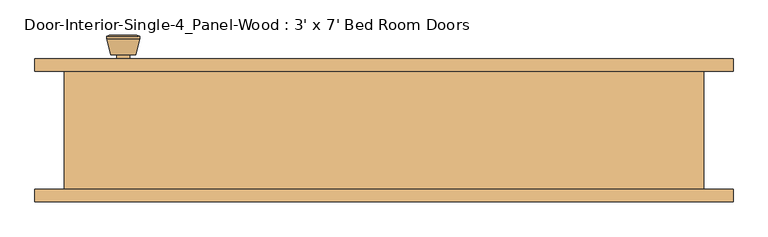
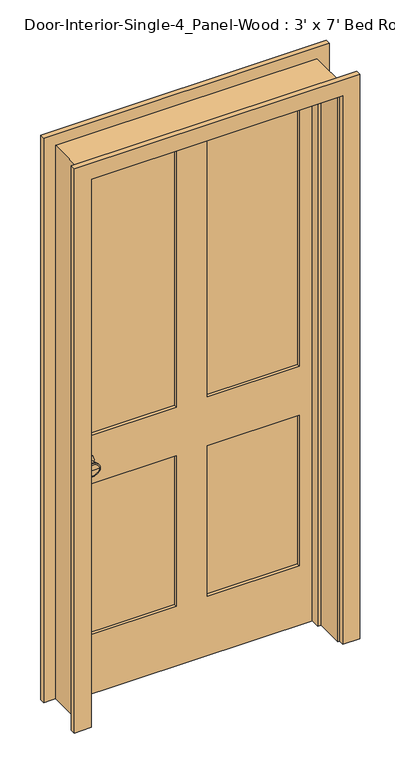
"""IFC4 building model written with IfcOpenShell, lengths in millimetres: door geometry, Door-Interior-Single-4_Panel-Wood : 3' x 7' Bed Room Doors."""

from ifc_helpers import new_model, si_unit, point, frame, frame_2d, origin, place, context, project, spatial, polyline, circle_curve, trimmed, segment, composite_curve, outline, extrude, faceted_brep, source, transform, mapped, element, save
from ifc_brep_helpers import plane_surface, cylinder_surface, revolved_surface, advanced_brep


def door_interior_single_4_panel_wood_3_x_7_bed_room_doors_9f8eaeea(model_context):
    return source(origin(), model_context, "Body", "SolidModel", [
        advanced_brep(
        [(-393.7, 44.8, 914.4), (-383.7, 44.8, 914.4), (-403.7, 44.8, 914.4), (-373.2241324, -4.2, 914.4), (-393.7, -4.2, 914.4), (-414.1758676, -4.2, 914.4), (-368.7, -2.3721319, 914.4), (-418.7, -2.3721319, 914.4), (-368.7, 1.0915463, 914.4), (-418.7, 1.0915463, 914.4), (-375.063764, 25.8, 914.4), (-412.336236, 25.8, 914.4), (-383.7, 25.8, 914.4), (-403.7, 25.8, 914.4)],
        [
            (0, 1),
            (1, 2, circle_curve(frame((-393.7, 44.8, 914.4), z_axis=(0.0, 1.0, 0.0), x_axis=(-1.0, 0.0, 0.0)), 10.0)),
            (2, 0),
            (2, 1, circle_curve(frame((-393.7, 44.8, 914.4), z_axis=(0.0, 1.0, 0.0), x_axis=(-1.0, 0.0, 0.0)), 10.0)),
            (3, 4),
            (4, 5),
            (5, 3, circle_curve(frame((-393.7, -4.2, 914.4), z_axis=(0.0, -1.0, 0.0), x_axis=(-1.0, 0.0, 0.0)), 20.4758676)),
            (3, 5, circle_curve(frame((-393.7, -4.2, 914.4), z_axis=(0.0, -1.0, 0.0), x_axis=(-1.0, 0.0, 0.0)), 20.4758676)),
            (6, 3),
            (5, 7),
            (7, 6, circle_curve(frame((-393.7, -2.3721319, 914.4), z_axis=(0.0, -1.0, 0.0), x_axis=(-1.0, 0.0, 0.0)), 25.0)),
            (6, 7, circle_curve(frame((-393.7, -2.3721319, 914.4), z_axis=(0.0, -1.0, 0.0), x_axis=(-1.0, 0.0, 0.0)), 25.0)),
            (8, 6),
            (7, 9),
            (9, 8, circle_curve(frame((-393.7, 1.0915463, 914.4), z_axis=(0.0, -1.0, 0.0), x_axis=(-1.0, 0.0, 0.0)), 25.0)),
            (8, 9, circle_curve(frame((-393.7, 1.0915463, 914.4), z_axis=(0.0, -1.0, 0.0), x_axis=(-1.0, 0.0, 0.0)), 25.0)),
            (10, 8),
            (9, 11),
            (11, 10, circle_curve(frame((-393.7, 25.8, 914.4), z_axis=(0.0, -1.0, 0.0), x_axis=(-1.0, 0.0, 0.0)), 18.636236)),
            (10, 11, circle_curve(frame((-393.7, 25.8, 914.4), z_axis=(0.0, -1.0, 0.0), x_axis=(-1.0, 0.0, 0.0)), 18.636236)),
            (12, 10),
            (11, 13),
            (13, 12, circle_curve(frame((-393.7, 25.8, 914.4), z_axis=(0.0, -1.0, 0.0), x_axis=(-1.0, 0.0, 0.0)), 10.0)),
            (12, 13, circle_curve(frame((-393.7, 25.8, 914.4), z_axis=(0.0, -1.0, 0.0), x_axis=(-1.0, 0.0, 0.0)), 10.0)),
            (1, 12),
            (13, 2),
        ],
        [
            plane_surface(frame((-393.7, 44.8, 914.4), z_axis=(0.0, 1.0, 0.0), x_axis=(-1.0, 0.0, 0.0))),
            plane_surface(frame((-393.7, -4.2, 914.4), z_axis=(0.0, -1.0, 0.0), x_axis=(-1.0, 0.0, 0.0))),
            revolved_surface(polyline([(-414.1758676, -4.2, 914.4), (-418.7, -2.3721319, 914.4)]), (-393.7, 44.8, 914.4), (0.0, 1.0, 0.0)),
            cylinder_surface(frame((-393.7, 44.8, 914.4), z_axis=(0.0, 1.0, 0.0), x_axis=(-1.0, 0.0, 0.0)), 25.0),
            revolved_surface(polyline([(-418.7, 1.0915463, 914.4), (-412.336236, 25.8, 914.4)]), (-393.7, 44.8, 914.4), (0.0, 1.0, 0.0)),
            plane_surface(frame((-393.7, 25.8, 914.4), z_axis=(0.0, 1.0, 0.0), x_axis=(-1.0, 0.0, 0.0))),
            cylinder_surface(frame((-393.7, 44.8, 914.4), z_axis=(0.0, 1.0, 0.0), x_axis=(-1.0, 0.0, 0.0)), 10.0),
        ],
        [
            (0, [[1, 2, 3]]),
            (0, [[-3, 4, -1]]),
            (1, [[5, 6, 7]]),
            (1, [[-6, -5, 8]]),
            (2, [[9, -7, 10, 11]]),
            (2, [[-10, -8, -9, 12]]),
            (3, [[13, -11, 14, 15]]),
            (3, [[-14, -12, -13, 16]]),
            (4, [[17, -15, 18, 19]]),
            (4, [[-18, -16, -17, 20]]),
            (5, [[21, -19, 22, 23]]),
            (5, [[-22, -20, -21, 24]]),
            (6, [[25, -23, 26, -2]]),
            (6, [[-26, -24, -25, -4]]),
        ],
    ),
        extrude(outline(composite_curve([segment(trimmed(circle_curve(frame_2d((914.4, -393.7)), 30.0), [point((914.4, -423.7))], [point((914.4, -363.7))], False, "CARTESIAN"), True, "CONTINUOUS"), segment(trimmed(circle_curve(frame_2d((914.4, -393.7)), 30.0), [point((914.4, -363.7))], [point((914.4, -423.7))], False, "CARTESIAN"), True, "CONTINUOUS")], self_intersect=False)), frame((0.0, 44.8, 0.0), z_axis=(0.0, 1.0, 0.0), x_axis=(0.0, 0.0, 1.0)), (0.0, 0.0, 1.0), 6.0),
        advanced_brep(
        [(-393.7, 91.725, 914.4), (-403.7, 91.725, 914.4), (-383.7, 91.725, 914.4), (-373.2241324, 140.725, 914.4), (-414.1758676, 140.725, 914.4), (-393.7, 140.725, 914.4), (-368.7, 138.8971319, 914.4), (-418.7, 138.8971319, 914.4), (-368.7, 135.4334537, 914.4), (-418.7, 135.4334537, 914.4), (-375.063764, 110.725, 914.4), (-412.336236, 110.725, 914.4), (-383.7, 110.725, 914.4), (-403.7, 110.725, 914.4)],
        [
            (0, 1),
            (1, 2, circle_curve(frame((-393.7, 91.725, 914.4), z_axis=(0.0, -1.0, 0.0), x_axis=(-1.0, 0.0, 0.0)), 10.0)),
            (2, 0),
            (2, 1, circle_curve(frame((-393.7, 91.725, 914.4), z_axis=(0.0, -1.0, 0.0), x_axis=(-1.0, 0.0, 0.0)), 10.0)),
            (3, 4, circle_curve(frame((-393.7, 140.725, 914.4), z_axis=(0.0, 1.0, 0.0), x_axis=(-1.0, 0.0, 0.0)), 20.4758676)),
            (4, 5),
            (5, 3),
            (4, 3, circle_curve(frame((-393.7, 140.725, 914.4), z_axis=(0.0, 1.0, 0.0), x_axis=(-1.0, 0.0, 0.0)), 20.4758676)),
            (6, 7, circle_curve(frame((-393.7, 138.8971319, 914.4), z_axis=(0.0, 1.0, 0.0), x_axis=(-1.0, 0.0, 0.0)), 25.0)),
            (7, 4),
            (3, 6),
            (7, 6, circle_curve(frame((-393.7, 138.8971319, 914.4), z_axis=(0.0, 1.0, 0.0), x_axis=(-1.0, 0.0, 0.0)), 25.0)),
            (8, 9, circle_curve(frame((-393.7, 135.4334537, 914.4), z_axis=(0.0, 1.0, 0.0), x_axis=(-1.0, 0.0, 0.0)), 25.0)),
            (9, 7),
            (6, 8),
            (9, 8, circle_curve(frame((-393.7, 135.4334537, 914.4), z_axis=(0.0, 1.0, 0.0), x_axis=(-1.0, 0.0, 0.0)), 25.0)),
            (10, 11, circle_curve(frame((-393.7, 110.725, 914.4), z_axis=(0.0, 1.0, 0.0), x_axis=(-1.0, 0.0, 0.0)), 18.636236)),
            (11, 9),
            (8, 10),
            (11, 10, circle_curve(frame((-393.7, 110.725, 914.4), z_axis=(0.0, 1.0, 0.0), x_axis=(-1.0, 0.0, 0.0)), 18.636236)),
            (12, 13, circle_curve(frame((-393.7, 110.725, 914.4), z_axis=(0.0, 1.0, 0.0), x_axis=(-1.0, 0.0, 0.0)), 10.0)),
            (13, 11),
            (10, 12),
            (13, 12, circle_curve(frame((-393.7, 110.725, 914.4), z_axis=(0.0, 1.0, 0.0), x_axis=(-1.0, 0.0, 0.0)), 10.0)),
            (1, 13),
            (12, 2),
        ],
        [
            plane_surface(frame((-393.7, 91.725, 914.4), z_axis=(0.0, -1.0, 0.0), x_axis=(-1.0, 0.0, 0.0))),
            plane_surface(frame((-393.7, 140.725, 914.4), z_axis=(0.0, 1.0, 0.0), x_axis=(-1.0, 0.0, 0.0))),
            revolved_surface(polyline([(-414.1758676, 140.725, 914.4), (-418.7, 138.8971319, 914.4)]), (-393.7, 91.725, 914.4), (0.0, -1.0, 0.0)),
            cylinder_surface(frame((-393.7, 91.725, 914.4), z_axis=(0.0, -1.0, 0.0), x_axis=(-1.0, 0.0, 0.0)), 25.0),
            revolved_surface(polyline([(-418.7, 135.4334537, 914.4), (-412.336236, 110.725, 914.4)]), (-393.7, 91.725, 914.4), (0.0, -1.0, 0.0)),
            plane_surface(frame((-393.7, 110.725, 914.4), z_axis=(0.0, -1.0, 0.0), x_axis=(-1.0, 0.0, 0.0))),
            cylinder_surface(frame((-393.7, 91.725, 914.4), z_axis=(0.0, -1.0, 0.0), x_axis=(-1.0, 0.0, 0.0)), 10.0),
        ],
        [
            (0, [[1, 2, 3]]),
            (0, [[-3, 4, -1]]),
            (1, [[5, 6, 7]]),
            (1, [[8, -7, -6]]),
            (2, [[9, 10, -5, 11]]),
            (2, [[12, -11, -8, -10]]),
            (3, [[13, 14, -9, 15]]),
            (3, [[16, -15, -12, -14]]),
            (4, [[17, 18, -13, 19]]),
            (4, [[20, -19, -16, -18]]),
            (5, [[21, 22, -17, 23]]),
            (5, [[24, -23, -20, -22]]),
            (6, [[-2, 25, -21, 26]]),
            (6, [[-4, -26, -24, -25]]),
        ],
    ),
        extrude(outline(composite_curve([segment(trimmed(circle_curve(frame_2d((914.4, -393.7)), 30.0), [point((914.4, -423.7))], [point((914.4, -363.7))], False, "CARTESIAN"), True, "CONTINUOUS"), segment(trimmed(circle_curve(frame_2d((914.4, -393.7)), 30.0), [point((914.4, -363.7))], [point((914.4, -423.7))], False, "CARTESIAN"), True, "CONTINUOUS")], self_intersect=False)), frame((0.0, 85.725, 0.0), z_axis=(0.0, 1.0, 0.0), x_axis=(0.0, 0.0, 1.0)), (0.0, 0.0, 1.0), 6.0),
        faceted_brep([(482.6, 85.725, 0.0), (482.6, -92.075, 0.0), (457.2, -92.075, 0.0), (457.2, 15.875, 0.0), (444.5, 15.875, 0.0), (444.5, 50.8, 0.0), (457.2, 50.8, 0.0), (457.2, 85.725, 0.0), (482.6, 85.725, 2159.0), (482.6, -92.075, 2159.0), (-482.6, -92.075, 2159.0), (-482.6, -92.075, 0.0), (-457.2, -92.075, 0.0), (-457.2, -92.075, 2133.6), (457.2, -92.075, 2133.6), (457.2, 15.875, 2133.6), (-457.2, 15.875, 2133.6), (-457.2, 15.875, 0.0), (-444.5, 15.875, 0.0), (-444.5, 15.875, 2120.9), (444.5, 15.875, 2120.9), (444.5, 50.8, 2120.9), (-444.5, 50.8, 2120.9), (-444.5, 50.8, 0.0), (-457.2, 50.8, 0.0), (-457.2, 50.8, 2133.6), (457.2, 50.8, 2133.6), (457.2, 85.725, 2133.6), (-457.2, 85.725, 2133.6), (-457.2, 85.725, 0.0), (-482.6, 85.725, 0.0), (-482.6, 85.725, 2159.0)], [[[0, 1, 2, 3, 4, 5, 6, 7]], [[1, 0, 8, 9]], [[2, 1, 9, 10, 11, 12, 13, 14]], [[3, 2, 14, 15]], [[4, 3, 15, 16, 17, 18, 19, 20]], [[5, 4, 20, 21]], [[6, 5, 21, 22, 23, 24, 25, 26]], [[7, 6, 26, 27]], [[0, 7, 27, 28, 29, 30, 31, 8]], [[9, 8, 31, 10]], [[15, 14, 13, 16]], [[21, 20, 19, 22]], [[27, 26, 25, 28]], [[30, 29, 24, 23, 18, 17, 12, 11]], [[10, 31, 30, 11]], [[16, 13, 12, 17]], [[22, 19, 18, 23]], [[28, 25, 24, 29]]]),
        extrude(outline(polyline([(2133.6, -457.2), (0.0, -457.2), (0.0, 457.2), (2133.6, 457.2), (2133.6, -457.2)]), holes=[polyline([(2014.5375, 57.15), (2014.5375, 396.875), (1009.65, 396.875), (1009.65, 57.15), (2014.5375, 57.15)]), polyline([(1009.65, -57.15), (1009.65, -396.875), (2014.5375, -396.875), (2014.5375, -57.15), (1009.65, -57.15)]), polyline([(819.15, 57.15), (819.15, 396.875), (231.775, 396.875), (231.775, 57.15), (819.15, 57.15)]), polyline([(231.775, -57.15), (231.775, -396.875), (819.15, -396.875), (819.15, -57.15), (231.775, -57.15)])]), frame((0.0, 50.8, 0.0), z_axis=(0.0, 1.0, 0.0), x_axis=(0.0, 0.0, 1.0)), (0.0, 0.0, 1.0), 34.925),
        extrude(outline(polyline([(396.875, 62.4416667), (57.15, 62.4416667), (57.15, 74.0833333), (396.875, 74.0833333), (396.875, 62.4416667)])), frame((0.0, 0.0, 1009.65), z_axis=(0.0, 0.0, 1.0), x_axis=(1.0, 0.0, 0.0)), (0.0, 0.0, 1.0), 1004.8875),
        extrude(outline(polyline([(-57.15, 62.4416667), (-396.875, 62.4416667), (-396.875, 74.0833333), (-57.15, 74.0833333), (-57.15, 62.4416667)])), frame((0.0, 0.0, 1009.65), z_axis=(0.0, 0.0, 1.0), x_axis=(1.0, 0.0, 0.0)), (0.0, 0.0, 1.0), 1004.8875),
        extrude(outline(polyline([(396.875, 62.4416667), (57.15, 62.4416667), (57.15, 74.0833333), (396.875, 74.0833333), (396.875, 62.4416667)])), frame((0.0, 0.0, 231.775), z_axis=(0.0, 0.0, 1.0), x_axis=(1.0, 0.0, 0.0)), (0.0, 0.0, 1.0), 587.375),
        extrude(outline(polyline([(-57.15, 62.4416667), (-396.875, 62.4416667), (-396.875, 74.0833333), (-57.15, 74.0833333), (-57.15, 62.4416667)])), frame((0.0, 0.0, 231.775), z_axis=(0.0, 0.0, 1.0), x_axis=(1.0, 0.0, 0.0)), (0.0, 0.0, 1.0), 587.375),
        extrude(outline(polyline([(0.0, 463.55), (0.0, 527.05), (2203.45, 527.05), (2203.45, -527.05), (0.0, -527.05), (0.0, -463.55), (2139.95, -463.55), (2139.95, 463.55), (0.0, 463.55)])), frame((0.0, 85.725, 0.0), z_axis=(0.0, 1.0, 0.0), x_axis=(0.0, 0.0, 1.0)), (0.0, 0.0, 1.0), 19.05),
        extrude(outline(polyline([(0.0, 463.55), (0.0, 527.05), (2203.45, 527.05), (2203.45, -527.05), (0.0, -527.05), (0.0, -463.55), (2139.95, -463.55), (2139.95, 463.55), (0.0, 463.55)])), frame((0.0, -111.125, 0.0), z_axis=(0.0, 1.0, 0.0), x_axis=(0.0, 0.0, 1.0)), (0.0, 0.0, 1.0), 19.05),
    ])


if __name__ == "__main__":
    model = new_model("IFC4")
    model_context = context("Model", 3, world=origin())
    ifc_project = project(units=[si_unit("LENGTHUNIT", "METRE", prefix="MILLI")], contexts=[model_context])
    site = spatial("IfcSite", under=ifc_project)
    building = spatial("IfcBuilding", under=site)
    placement = place(None, origin())
    door_interior_single_4_panel_wood_3_x_7_bed_room_doors_shape = door_interior_single_4_panel_wood_3_x_7_bed_room_doors_9f8eaeea(model_context)
    element("IfcDoor", 1, ObjectType="Door-Interior-Single-4_Panel-Wood : 3' x 7' Bed Room Doors", at=placement, inside=building, context=model_context, shape_type="MappedRepresentation", body=[
        mapped(door_interior_single_4_panel_wood_3_x_7_bed_room_doors_shape, transform((0.0, 0.0, 0.0), x_axis=(1.0, 0.0, 0.0), y_axis=(0.0, 1.0, 0.0), z_axis=(0.0, 0.0, 1.0))),
    ])
    save(model, "model.ifc")

# Revit data of these elements
# Type "Door-Interior-Single-4_Panel-Wood : 3' x 7' Bed Room Doors"
#   Type Mark = "13"
#   Assembly Code = "C1020300"
#   Analytic Construction = "Wooden"
#   Top Rail = 0' - 4 11/16"
#   Thickness = 0' - 1 3/8"
#   Thermal Resistance (R) = 2.5876 (h·ft²·°F)/BTU
#   Swing Angle [instance default] = 90.00°
#   Stiles = 0' - 2 3/8"
#   Rough Width = 3' - 2"
#   Rough Height = 7' - 1"
#   Mullion = 0' - 4 1/2"
#   Lock Rail = 0' - 7 1/2"
#   Height = 7' - 0"
#   Width = 3' - 0"
#   Heat Transfer Coefficient (U) = 0.3865 BTU/(h·ft²·°F)
#   Bottom Rail = 0' - 9 1/8"
#   Trim Material = Cherry
#   Panel Material = Cherry
#   Frame Material = Cherry
#   Door Handle Material = Aluminum
#   Visual Light Transmittance = 0
#   Solar Heat Gain Coefficient = 0
#   Wall Closure = (empty or 0)
#   Function = (empty or 0)
# Element 1 (IfcDoor, "Door-Interior-Single-4_Panel-Wood : 3' x 7' Bed Room Doors")
#   Materials on its faces: "Cherry", "Aluminum"
# Materials
#   "Cherry": class "Wood", colour RGB 226 177 128, transparency 0, Description = "Prunus Serotina", Cost = 0
#   "Aluminum": class "Metal", colour RGB 247 247 247, transparency 0, Description = "Aluminum 6061", Cost = 0
